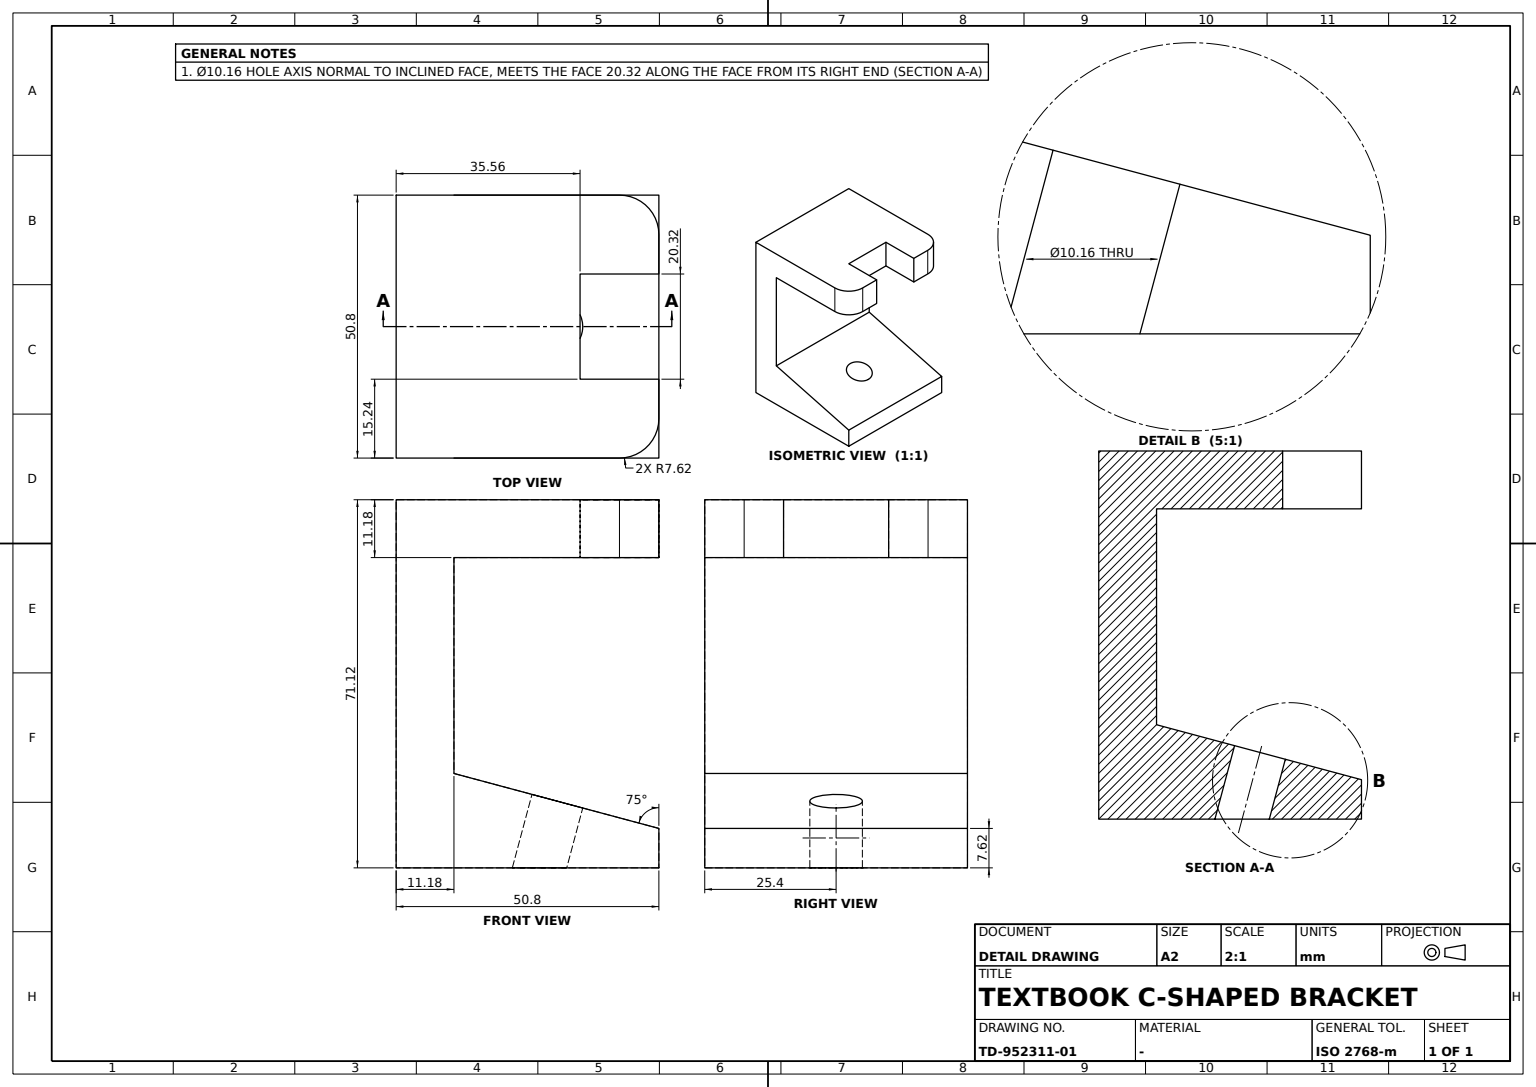
CATIA V5 part; units mm, degrees
sketch "Sketch1" plane through (0, 0, 0) normal (0, 1, 0) x (-1, 0, 0)
  line L0 (0, 0) -> (0, 71.12)
  line L1 (0, 71.12) -> (-50.8, 71.12)
  line L2 (-50.8, 71.12) -> (-50.8, 59.944)
  line L3 (-50.8, 59.944) -> (-11.176, 59.944)
  line L4 (-11.176, 59.944) -> (-11.176, 18.2372)
  line L5 (-11.176, 18.2372) -> (-50.8, 7.62)
  point P0 (-50.8, 7.62)
  line L6 (-50.8, 7.62) -> (-50.8, 0)
  point P1 (-50.8, 0)
  line L7 (-50.8, 0) -> (0, 0)
  dimension "length L6" = 7.62
  dimension "length L0" = 71.12
  dimension "D3" = 11.176
  dimension "length L2" = 11.176
  dimension "D5" = 15
  dimension "length L1" = 50.8
  constraint vertical L0 y-axis
  constraint vertical L2 y-axis
  constraint vertical L4 y-axis
  constraint vertical L6 y-axis
  constraint horizontal L1 x-axis
  constraint horizontal L3 x-axis
  constraint horizontal L7 x-axis
  constraint coincidence P0 L2
  constraint coincidence P1 x-axis
extrude "Pad1" add sketch "Sketch1" along normal mid plane 50.8
sketch "Sketch2" plane through (0, 0, 71.12) normal (0, 0, 1) x (1, 0, 0)
  line L0 (35.56, 10.16) -> (50.8, 10.16)
  line L1 (50.8, 10.16) -> (50.8, -10.16)
  line L2 (50.8, -10.16) -> (35.56, -10.16)
  line L3 (35.56, -10.16) -> (35.56, 10.16)
  line L4 (50.8, -25.4) -> (50.8, 25.4) construction
  line L5 (0, -25.4) -> (0, 25.4) construction
  line L6 (0, -25.4) -> (50.8, -25.4) construction
  dimension "length L1" = 20.32
  dimension "distance L3 L5" = 35.56
  dimension "distance L2 L6" = 15.24
  constraint horizontal L0 x-axis
  constraint horizontal L2 x-axis
  constraint vertical L1 y-axis
  constraint vertical L3 y-axis
  constraint coincidence L1 L4
extrude "Pocket1" cut sketch "Sketch2" against normal up to next
fillet "Fillet1" radius 7.62 2 edges at (50.8, -25.4, 65.532) (50.8, 25.4, 65.532)
sketch "Sketch3" plane through (5.308, 0, 19.8095) normal (0.2588, 0, 0.9659) x (0, 1, 0)
  circle A0 centre (0, -26.7768) radius 5.08
  point P0 (0, -26.7768)
  line L0 (25.4, -6.075) -> (25.4, -47.0968) construction
  line L1 (-25.4, -47.0968) -> (25.4, -47.0968) construction
  dimension "distance P0 L0" = 25.4
  dimension "radius A0" = 5.08
  dimension "distance P0 L1" = 20.32
extrude "Pocket2" cut sketch "Sketch3" against normal up to next
properties part number "catia 31"
